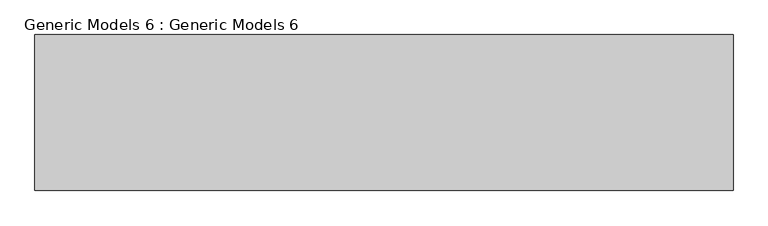
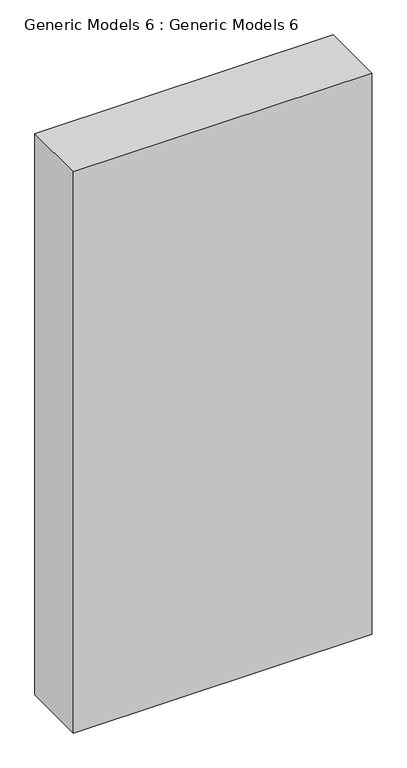
"""IFC4 building model written with IfcOpenShell, lengths in millimetres: proxy geometry, Generic Models 6 : Generic Models 6."""

from ifc_helpers import new_model, si_unit, frame, origin, place, context, project, spatial, polyline, outline, extrude, source, transform, mapped, element, save


def generic_models_6_generic_models_6_03283b1a(model_context):
    return source(origin(), model_context, "Body", "SweptSolid", [
        extrude(outline(polyline([(9548.0374104, -8641.1821053), (9548.0374104, -9854.1879232), (4118.5117887, -9854.1879232), (4118.5117887, -8641.1821053), (9548.0374104, -8641.1821053)])), frame((0.0, 0.0, 2083.8939548), z_axis=(0.0, 0.0, 1.0), x_axis=(1.0, 0.0, 0.0)), (0.0, 0.0, 1.0), 10793.9060452),
    ])


if __name__ == "__main__":
    model = new_model("IFC4")
    model_context = context("Model", 3, world=origin())
    ifc_project = project(units=[si_unit("LENGTHUNIT", "METRE", prefix="MILLI")], contexts=[model_context])
    site = spatial("IfcSite", under=ifc_project)
    building = spatial("IfcBuilding", under=site)
    placement = place(None, origin())
    generic_models_6_generic_models_6_shape = generic_models_6_generic_models_6_03283b1a(model_context)
    element("IfcBuildingElementProxy", 1, Name="Generic Models 6 : Generic Models 6", ObjectType="Generic Models 6 : Generic Models 6", at=placement, inside=building, context=model_context, shape_type="MappedRepresentation", body=[
        mapped(generic_models_6_generic_models_6_shape, transform((0.0, 0.0, 0.0), x_axis=(1.0, 0.0, 0.0), y_axis=(0.0, 1.0, 0.0), z_axis=(0.0, 0.0, 1.0))),
    ])
    save(model, "model.ifc")
